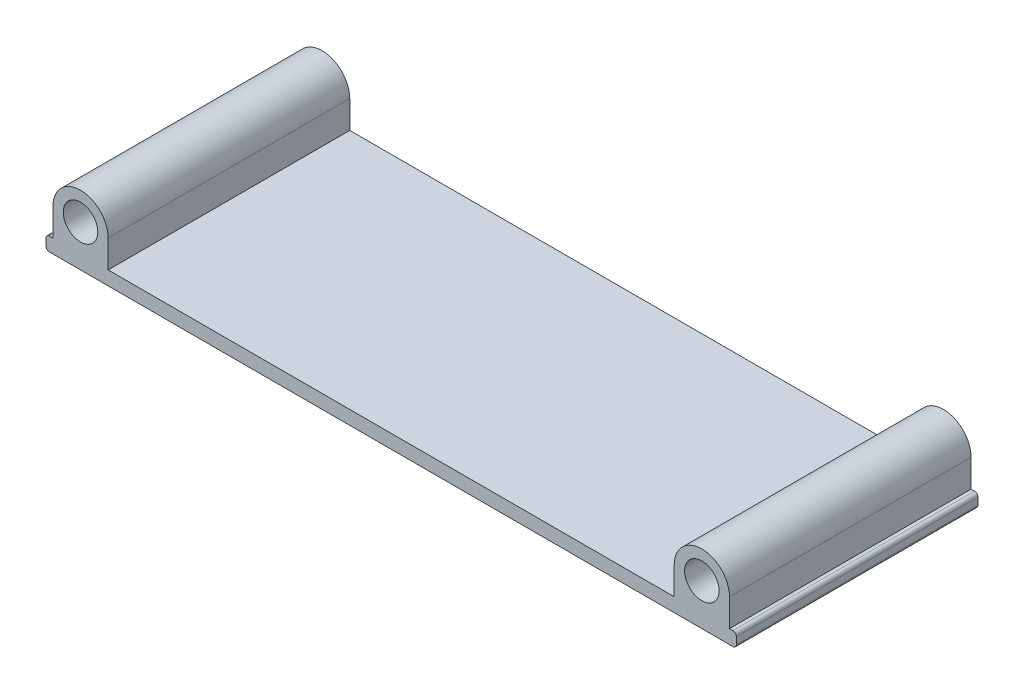
SolidWorks part; units mm, degrees
material "Plain Carbon Steel"
ref_plane "Front Plane" through (0, 0, 0) normal (0, 0, 1) x (1, 0, 0)
ref_plane "Top Plane" through (0, 0, 0) normal (0, 1, 0) x (1, 0, 0)
ref_plane "Right Plane" through (0, 0, 0) normal (1, 0, 0) x (0, 0, -1)
sketch "Rolled Edge Plate Profile" plane through (0, 0, 0) normal (0, 0, 1) x (1, 0, 0)
  line L0 (-45, -3) -> (-45, 5) construction
  line L1 (-50, 1) -> (50, 1)
  line L2 (-50, 1) -> (-50, -1)
  line L3 (-50, -1) -> (50, -1)
  line L4 (50, 1) -> (50, -1)
  line L5 (-50, 1) -> (50, -1) construction
  line L6 (-50, -1) -> (50, 1) construction
  line L7 (-49, -3) -> (-49, 5)
  line L8 (-41, -3) -> (-41, 5)
  line L9 (45, -3) -> (45, 5) construction
  line L10 (41, -3) -> (41, 5)
  line L11 (49, -3) -> (49, 5)
  arc A0 (-49, -3) -> (-41, -3) centre (-45, -3) ccw
  arc A1 (-41, 5) -> (-49, 5) centre (-45, 5) ccw
  arc A2 (41, -3) -> (49, -3) centre (45, -3) ccw
  arc A3 (49, 5) -> (41, 5) centre (45, 5) ccw
  circle A4 centre (45, 5) radius 2.5
  circle A5 centre (-45, 5) radius 2.5
  point P0 (0, 0)
  point P8 (-45, 1)
  point P14 (45, 1)
  dimension "D7" = 4
  dimension "D8" = 5
  dimension "D9" = 4
  dimension "D1" = 100
  dimension "D2" = 2
  dimension "D3" = 4
  dimension "D4" = 4
  dimension "D5" = 5
  dimension "D6" = 5
extrude "Plate Extrude 35mm" add sketch "Rolled Edge Plate Profile" along normal mid plane 35 contours L11 A3 L10 L1 A4 | L3 L10 L1 L8 | L11 L3 L4 L1 | L3 L11 L1 L10 | L3 L8 L1 L7 | L3 L7 L1 L2 | L8 A1 L7 L1 A5
fillet "Edge Fillets R0.5" radius 0.5 4 edges at (50, -1, 0) (50, 1, 0) (-50, -1, 0) (-50, 1, 0)
